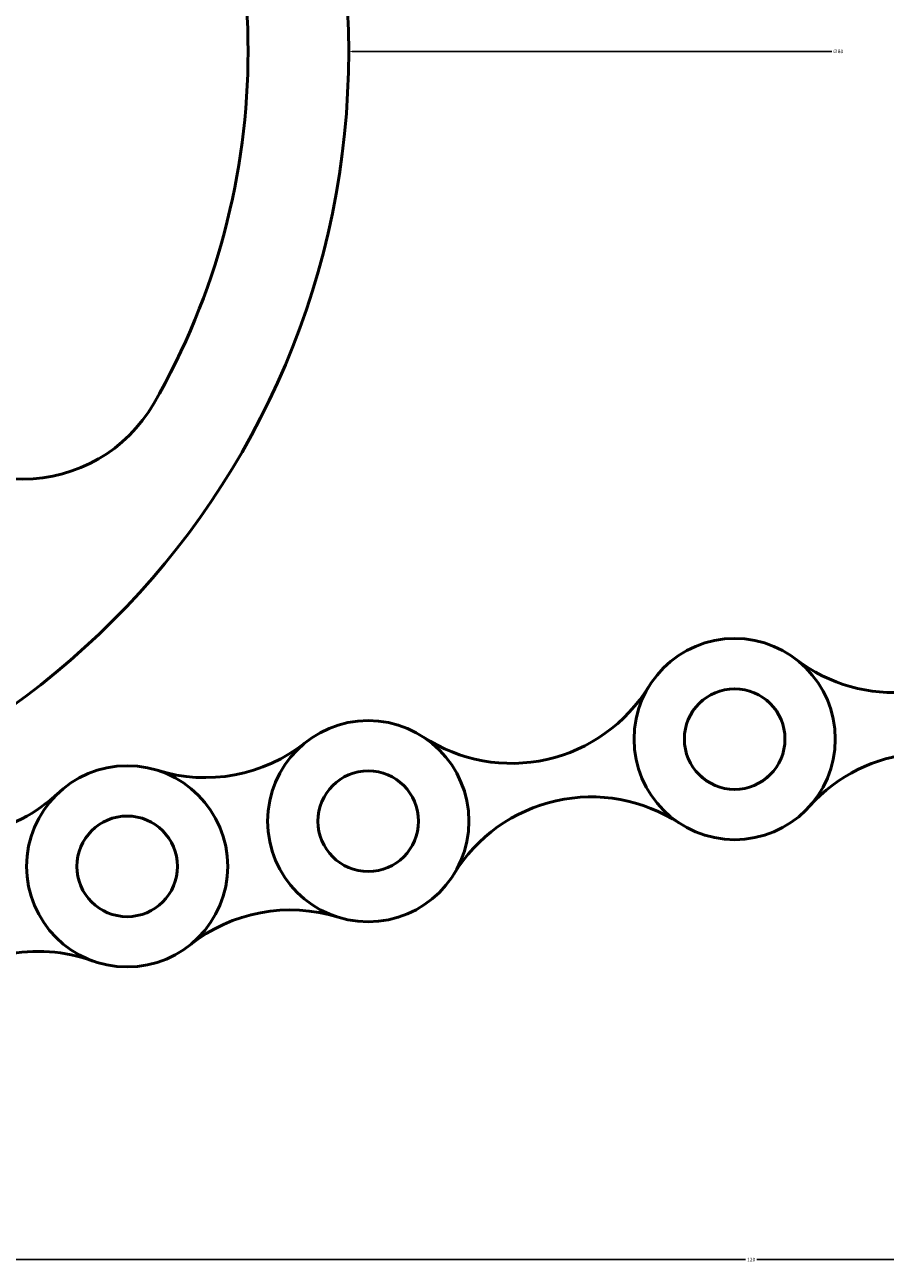
# Model space of a CAD drawing. Units: inches. Extents: x 413 to 622, y 326 to 447.
# Tile 8 of 15: x 497 to 539, y 326 to 388. Entities that reach past the tile are written whole.
import ezdxf

# ---------------------------------------------------------------- set-up
doc = ezdxf.new("R2010")
doc.units = ezdxf.units.IN
doc.header["$MEASUREMENT"] = 0
doc.layers.add('M-DIMS', color=2, linetype='Continuous', lineweight=18)
doc.layers.add('M-OUTL', color=7, linetype='Continuous', lineweight=50)
doc.styles.get("Standard").update_dxf_attribs({"font": 'arial.ttf'})
doc.dimstyles.get("Standard").update_dxf_attribs({"dimtxt": 0.18, "dimasz": 0.18, "dimexe": 0.18, "dimexo": 0.0625, "dimgap": 0.09, "dimtad": 0, "dimtih": 1, "dimtoh": 1, "dimdec": 4, "dimzin": 0, "dimdsep": 46, "dimtxsty": 'Standard', "dimcen": 0.09, "dimadec": 0, "dimazin": 0, "dimtfac": 1, "dimtdec": 4, "dimtofl": 0, "dimtmove": 0, "dimatfit": 3, "dimfxl": 1, "dimtolj": 1, "dimtzin": 0, "dimarcsym": 0})

# ---------------------------------------------------------------- blocks, each defined once
blk = doc.blocks.new('CHAIN-ROLLER-PIN')
for radius in [5, 2.5]:
    blk.add_circle((5, 5), radius)
blk = doc.blocks.new('SPROCKET-WEB-SLOT')
for centre, radius, start, end in [((7.501, 21.25), 7.5, 30, 210), ((31.317, 35), 35, 210, 270)]:
    blk.add_arc(centre, radius, start, end)
blk = doc.blocks.new('CHAIN-LINK-WAIST-P13_603')
for centre, start, end in [((7.205, 15.87), 226.77186, 289.86266), ((2.718, -5.829), 46.77186, 109.86266)]:
    blk.add_arc(centre, 8, start, end)
blk = doc.blocks.new('CHAIN-LINK-WAIST-P12_188')
for centre, start, end in [((6.613, 16.319), 231.4363, 287.34282), ((2.384, -6.255), 51.4363, 107.34282)]:
    blk.add_arc(centre, 8, start, end)
blk = doc.blocks.new('CHAIN-LINK-WAIST-P18_660')
for centre, start, end in [((8.344, 13.487), 211.50374, 303.22962), ((4.384, -4.18), 31.50374, 123.22962)]:
    blk.add_arc(centre, 8, start, end)
blk = doc.blocks.new('CHAIN-LINK-WAIST-P17_664')
for centre, start, end in [((6.624, 13.651), 221.93853, 307.52912), ((4.873, -5.347), 41.93853, 127.52912)]:
    blk.add_arc(centre, 8, start, end)
blk = doc.blocks.new('*D11')
at = {"layer": 'Defpoints', "color": 0, "transparency": 16777216}
for p in [(621.66, 446.422), (621.66, 388.074), (423.314, 378.888)]:
    blk.add_point(p, dxfattribs=at)
at = {"layer": 'M-DIMS', "color": 0, "lineweight": -2, "transparency": 16777216}
for p, q in [((423.314, 378.95), (423.314, 446.602)), ((423.494, 446.422), (522.031, 446.422)), ((621.48, 446.422), (522.943, 446.422)), ((621.66, 388.137), (621.66, 446.602))]:
    blk.add_line(p, q, dxfattribs=at)
at = {"layer": 'M-DIMS', "color": 0, "transparency": 16777216}
for points in [[(423.494, 446.452), (423.494, 446.392), (423.314, 446.422)], [(621.48, 446.452), (621.48, 446.392), (621.66, 446.422)]]:
    blk.add_solid(points, dxfattribs=at)
at = {"layer": 'M-DIMS', "color": 0, "transparency": 16777216, "insert": (522.487, 446.422), "char_height": 0.18, "attachment_point": 5}
blk.add_mtext('\\A1;198.35', dxfattribs=at)
blk = doc.blocks.new('*D12')
at = {"layer": 'Defpoints', "color": 0, "transparency": 16777216}
for p in [(472.684, 386.392), (592.684, 386.392), (592.684, 326.361)]:
    blk.add_point(p, dxfattribs=at)
at = {"layer": 'M-DIMS', "color": 0, "lineweight": -2, "transparency": 16777216}
for p, q in [((472.684, 386.329), (472.684, 326.181)), ((592.684, 386.329), (592.684, 326.181)), ((472.864, 326.361), (532.404, 326.361)), ((592.504, 326.361), (532.964, 326.361))]:
    blk.add_line(p, q, dxfattribs=at)
at = {"layer": 'M-DIMS', "color": 0, "transparency": 16777216}
for points in [[(472.864, 326.391), (472.864, 326.331), (472.684, 326.361)], [(592.504, 326.391), (592.504, 326.331), (592.684, 326.361)]]:
    blk.add_solid(points, dxfattribs=at)
at = {"layer": 'M-DIMS', "color": 0, "transparency": 16777216, "insert": (532.684, 326.361), "char_height": 0.18, "attachment_point": 5}
blk.add_mtext('\\A1;120', dxfattribs=at)
blk = doc.blocks.new('*D24')
at = {"layer": 'Defpoints', "color": 0, "transparency": 16777216}
for p in [(432.684, 386.391), (512.684, 386.392)]:
    blk.add_point(p, dxfattribs=at)
at = {"layer": 'M-DIMS', "color": 0, "lineweight": -2, "transparency": 16777216}
for p, q in [((472.684, 386.302), (472.684, 386.482)), ((472.594, 386.392), (472.774, 386.392)), ((536.684, 386.392), (512.864, 386.392))]:
    blk.add_line(p, q, dxfattribs=at)
at = {"layer": 'M-DIMS', "color": 0, "transparency": 16777216}
blk.add_solid([(512.864, 386.422), (512.864, 386.362), (512.684, 386.392)], dxfattribs=at)
at = {"layer": 'M-DIMS', "color": 0, "transparency": 16777216, "insert": (537, 386.392), "char_height": 0.18, "attachment_point": 5}
blk.add_mtext('\\A1;∅80', dxfattribs=at)

msp = doc.modelspace()

# ---------------------------------------------------------------- linework, layer by layer
at = {"layer": 'M-OUTL'}
for centre, radius in [((472.6836, 386.3915), 40), ((531.863, 352.2242), 2.5)]:
    msp.add_circle(centre, radius, dxfattribs=at)

# ---------------------------------------------------------------- block references
for name, p, rotation in [('SPROCKET-WEB-SLOT', (518.6523, 376.7703), 119.9999999999996), ('CHAIN-LINK-WAIST-P17_664', (545.5506, 358.1679), 190.5323476777275), ('CHAIN-LINK-WAIST-P18_660', (526.5282, 357.1082), 205.2666329713933), ('CHAIN-LINK-WAIST-P12_188', (505.2934, 340.7021), 21.22088197134511), ('CHAIN-LINK-WAIST-P13_603', (492.4518, 337.9457), 23.36547829356988)]:
    msp.add_blockref(name, p, dxfattribs=dict(at, rotation=rotation))
for p in [(526.8634, 347.2247), (508.6556, 343.1437), (496.6765, 340.8996)]:
    msp.add_blockref('CHAIN-ROLLER-PIN', p, dxfattribs=at)

# ---------------------------------------------------------------- dimensions: what is measured, and where the dimension line sits
at = {"layer": 'M-DIMS'}
for base, p1, p2, override, picture, middle in [((621.66, 446.422), (423.3136, 378.8878), (621.66, 388.0741), {"dimdec": 2, "dimlfac": 1, "dimrnd": 0, "dimzin": 0, "dimdsep": 46, "dimlunit": 2}, '*D11', (522.4868, 446.422)), ((592.6836, 326.361), (472.6836, 386.3915), (592.6836, 386.3915), {"dimdec": 0, "dimlfac": 1, "dimrnd": 0, "dimzin": 0, "dimdsep": 46, "dimlunit": 2}, '*D12', (532.6836, 326.361))]:
    dim = msp.add_linear_dim(base=base, p1=p1, p2=p2, dimstyle='Standard', override=override, dxfattribs=at)
    dim.commit()
    dim.dimension.update_dxf_attribs({"geometry": picture, "text_midpoint": middle})
dim = msp.add_diameter_dim_2p(p1=(432.6836, 386.391), p2=(512.6836, 386.392), dimstyle='Standard', override={"dimdec": 0, "dimlfac": 1, "dimrnd": 0, "dimzin": 0, "dimdsep": 46, "dimlunit": 2}, dxfattribs=at)
dim.commit()
dim.dimension.update_dxf_attribs({"geometry": '*D24', "text_midpoint": (536.6836, 386.3923), "dimtype": 163})

doc.saveas('drawing.dxf')
